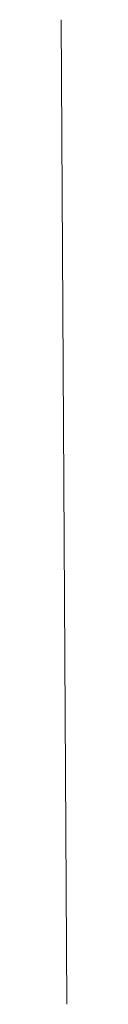
# Model space of a CAD drawing. Units: millimetres. Extents: x 9.37 to 9.4, y 393.17 to 398.84.
import ezdxf

# ---------------------------------------------------------------- set-up
doc = ezdxf.new("R2010")
doc.units = ezdxf.units.MM
doc.layers.add('M-CONS', color=8, linetype='Continuous', lineweight=13)

msp = doc.modelspace()

# ---------------------------------------------------------------- linework, layer by layer
at = {"layer": 'M-CONS', "extrusion": (1, 0, 0)}
msp.add_line((9.3654, 398.8399, 4.8393), (9.3984, 393.1704, 4.5822), dxfattribs=at)

doc.saveas('drawing.dxf')
